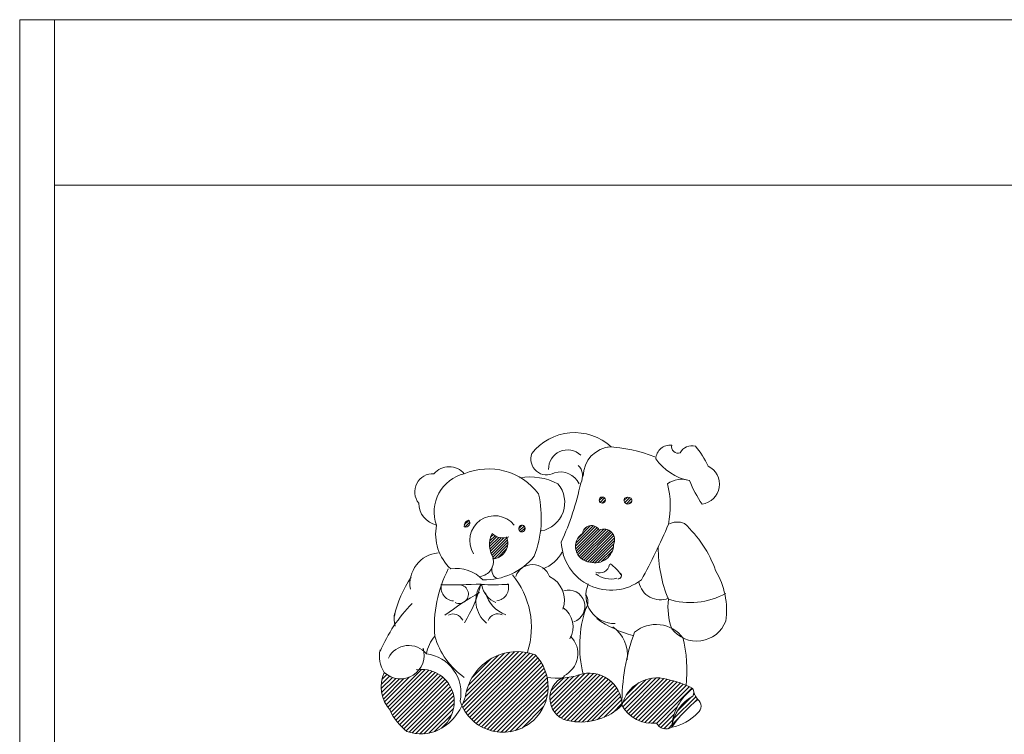
# Model space of a CAD drawing. Units: inches. Extents: x -17 to 1735, y -531 to 60.
# Tile 13 of 27: x 1734.65811 to 1734.68152, y -150.18312 to -150.16612. Entities that reach past the tile are written whole.
import ezdxf

# ---------------------------------------------------------------- set-up
doc = ezdxf.new("R2010")
doc.units = ezdxf.units.IN
doc.header["$MEASUREMENT"] = 0
doc.layers.add('A-FURN', color=242, linetype='Continuous', lineweight=18, true_color=0xcd2027)

# ---------------------------------------------------------------- blocks, each defined once
blk = doc.blocks.new('childrens_room_2')
for p, q in [((69.73591, 55.43419), (69.73591, 52.93419)), ((69.73591, 55.43419), (71.79591, 55.43419)), ((69.75691, 55.43419), (69.75691, 52.93419)), ((69.75691, 55.33419), (71.77791, 55.33419)), ((70.08595, 55.14364), (70.08806, 55.14576)), ((70.08652, 55.14255), (70.08916, 55.14519)), ((70.10093, 55.14362), (70.10296, 55.14564)), ((70.10141, 55.14243), (70.10447, 55.14548)), ((70.10235, 55.1417), (70.10548, 55.14483)), ((70.08769, 55.14205), (70.08967, 55.14404)), ((70.10389, 55.14157), (70.10561, 55.14328)), ((70.00446, 55.1289), (70.00723, 55.13166)), ((70.00492, 55.12768), (70.00776, 55.13053)), ((70.03738, 55.12677), (70.0394, 55.1288)), ((70.03775, 55.12548), (70.04054, 55.12827)), ((70.03867, 55.12473), (70.04115, 55.12721)), ((70.07163, 55.11599), (70.08361, 55.12796)), ((70.07175, 55.11443), (70.08464, 55.12732)), ((70.07184, 55.11786), (70.08237, 55.12839)), ((70.07284, 55.12053), (70.08079, 55.12848)), ((70.07662, 55.12598), (70.07827, 55.12763)), ((70.01971, 55.11745), (70.02412, 55.12186)), ((70.01974, 55.11582), (70.02535, 55.12142)), ((70.01987, 55.11928), (70.02302, 55.12243)), ((70.01993, 55.11433), (70.02673, 55.12114)), ((70.02024, 55.11297), (70.02833, 55.12106)), ((70.02037, 55.12145), (70.02202, 55.1231)), ((70.02064, 55.11171), (70.03014, 55.12121)), ((70.07206, 55.11308), (70.08548, 55.1265)), ((70.07253, 55.11188), (70.08674, 55.12609)), ((70.07312, 55.1108), (70.08874, 55.12642)), ((70.07383, 55.10984), (70.09025, 55.12625)), ((70.07464, 55.10898), (70.09149, 55.12583)), ((70.07555, 55.10823), (70.09255, 55.12522)), ((70.07658, 55.10758), (70.09344, 55.12445)), ((70.07772, 55.10706), (70.09419, 55.12353)), ((70.079, 55.10667), (70.09477, 55.12244)), ((70.08044, 55.10644), (70.09516, 55.12116)), ((70.02114, 55.11053), (70.0305, 55.1199)), ((70.02171, 55.10944), (70.03068, 55.11841)), ((70.02243, 55.10849), (70.0306, 55.11666)), ((70.08181, 55.10614), (70.09527, 55.1196)), ((70.08336, 55.10602), (70.09478, 55.11744)), ((70.08515, 55.10614), (70.09452, 55.11551)), ((70.02471, 55.10911), (70.02999, 55.11438)), ((70.08741, 55.10673), (70.09393, 55.11325)), ((70.00357, 55.01855), (70.03738, 55.05235)), ((70.00375, 55.02125), (70.03481, 55.05232)), ((70.00448, 55.01691), (70.03976, 55.0522)), ((70.00503, 55.02507), (70.032, 55.05204)), ((70.00547, 55.01537), (70.04198, 55.05189)), ((70.00579, 55.02836), (70.02885, 55.05142)), ((70.00655, 55.01392), (70.04408, 55.05145)), ((70.00696, 55.03206), (70.02515, 55.05025)), ((70.00771, 55.01255), (70.04605, 55.0509)), ((70.00896, 55.01127), (70.04771, 55.05002)), ((70.00938, 55.03701), (70.0202, 55.04783)), ((70.01029, 55.01007), (70.04888, 55.04866)), ((70.01171, 55.00895), (70.04997, 55.04722)), ((70.01321, 55.00793), (70.05097, 55.04569)), ((70.0148, 55.00698), (70.05189, 55.04407)), ((69.95473, 55.03553), (69.95771, 55.03851)), ((69.95583, 55.03916), (69.9563, 55.03963)), ((69.95722, 55.0203), (69.97853, 55.0416)), ((69.95821, 55.01876), (69.98093, 55.04148)), ((69.95932, 55.01733), (69.98309, 55.04111)), ((69.96023, 55.01571), (69.98506, 55.04055)), ((69.96111, 55.01406), (69.98688, 55.03983)), ((69.96207, 55.01249), (69.98855, 55.03896)), ((69.9631, 55.01099), (69.99009, 55.03798)), ((70.01649, 55.00614), (70.05271, 55.04237)), ((70.01827, 55.00539), (70.05343, 55.04056)), ((70.02017, 55.00476), (70.05405, 55.03863)), ((70.05654, 55.02088), (70.07405, 55.03838)), ((70.05717, 55.01897), (70.07735, 55.03916)), ((70.058, 55.01727), (70.08008, 55.03935)), ((70.05901, 55.01575), (70.08247, 55.03921)), ((70.06019, 55.0144), (70.08462, 55.03883)), ((70.06153, 55.01321), (70.08658, 55.03826)), ((69.95431, 55.03004), (69.96104, 55.03678)), ((69.95433, 55.0326), (69.95928, 55.03755)), ((69.95455, 55.02775), (69.96302, 55.03622)), ((69.95499, 55.02566), (69.96527, 55.03594)), ((69.9556, 55.02374), (69.96793, 55.03607)), ((69.95635, 55.02195), (69.97143, 55.03704)), ((69.96421, 55.00956), (69.99151, 55.03687)), ((69.96539, 55.00821), (69.99282, 55.03564)), ((69.96664, 55.00693), (69.99401, 55.0343)), ((69.96796, 55.00572), (69.99508, 55.03284)), ((70.02219, 55.00425), (70.05453, 55.03659)), ((70.02436, 55.00388), (70.05488, 55.0344)), ((70.02669, 55.00368), (70.05506, 55.03205)), ((70.05618, 55.02305), (70.07051, 55.03737)), ((70.0562, 55.0256), (70.06735, 55.03675)), ((70.05692, 55.02884), (70.06447, 55.0364)), ((70.06304, 55.01219), (70.08839, 55.03753)), ((70.06474, 55.01135), (70.09005, 55.03666)), ((70.06663, 55.01071), (70.09158, 55.03566)), ((70.06879, 55.01034), (70.09299, 55.03454)), ((70.07104, 55.01005), (70.09429, 55.0333)), ((70.07339, 55.00987), (70.09547, 55.03195)), ((70.10011, 55.02141), (70.11424, 55.03554)), ((70.10025, 55.01901), (70.11753, 55.03629)), ((70.10126, 55.01748), (70.1203, 55.03653)), ((70.10217, 55.02599), (70.10965, 55.03348)), ((70.10237, 55.01607), (70.12274, 55.03644)), ((70.10361, 55.01477), (70.12495, 55.03612)), ((70.10495, 55.01358), (70.127, 55.03563)), ((70.10641, 55.01251), (70.12905, 55.03515)), ((70.10798, 55.01155), (70.13105, 55.03462)), ((70.10968, 55.01072), (70.13299, 55.03403)), ((70.11152, 55.01002), (70.13489, 55.03339)), ((70.11352, 55.00949), (70.13673, 55.0327)), ((70.1157, 55.00914), (70.13853, 55.03197)), ((69.96935, 55.00458), (69.99604, 55.03126)), ((69.97108, 55.00377), (69.99686, 55.02955)), ((69.97306, 55.00322), (69.99753, 55.02769)), ((70.02923, 55.00369), (70.05502, 55.02948)), ((70.03206, 55.00399), (70.0547, 55.02663)), ((70.0759, 55.00985), (70.09653, 55.03048)), ((70.07861, 55.01003), (70.09746, 55.02888)), ((70.08158, 55.01047), (70.09827, 55.02716)), ((70.11813, 55.00904), (70.14027, 55.03118)), ((70.12069, 55.00907), (70.14198, 55.03036)), ((70.14276, 55.02607), (70.14348, 55.0268)), ((69.9752, 55.00283), (69.99804, 55.02567)), ((69.97754, 55.00264), (69.99834, 55.02344)), ((69.98012, 55.00268), (69.99838, 55.02095)), ((70.0353, 55.0047), (70.05395, 55.02335)), ((70.08492, 55.01128), (70.09892, 55.02528)), ((70.08888, 55.01271), (70.09941, 55.02323)), ((70.09436, 55.01565), (70.09968, 55.02097)), ((70.13088, 55.01166), (70.14436, 55.02514)), ((70.13299, 55.0163), (70.1418, 55.02511)), ((70.14358, 55.02183), (70.14541, 55.02366)), ((69.98305, 55.00308), (69.99803, 55.01806)), ((69.98657, 55.00407), (69.99694, 55.01444)), ((70.03934, 55.0062), (70.05241, 55.01927)), ((70.12175, 55.00759), (70.13309, 55.01893)), ((70.12317, 55.00648), (70.1313, 55.01461)), ((70.125, 55.00578), (70.13037, 55.01115)), ((70.12752, 55.00577), (70.1299, 55.00815)), ((70.13001, 55.00826), (70.13453, 55.01278))]:
    blk.add_line(p, q)
for centre, radius, start, end in [((70.07106, 55.15201), 0.03269, 47.56744, 142.1496), ((70.09417, 55.15831), 0.01786, 93.37661, 179.92184), ((70.08709, 55.08785), 0.08838, 68.42236, 87.41722), ((70.12888, 55.16833), 0.0088, 84.16796, 175.96386), ((70.13353, 55.17615), 0.00387, 165.93558, 290.16061), ((70.14204, 55.16872), 0.00811, 75.75386, 152.11841), ((70.10289, 55.14234), 0.05353, 24.30657, 39.76806), ((70.05427, 55.16875), 0.00962, 159.80669, 299.41128), ((70.06683, 55.16286), 0.01141, 45.88233, 182.2692), ((70.14635, 55.18708), 0.0319, 214.63102, 259.38614), ((69.99532, 55.15207), 0.01202, 40.3254, 139.6746), ((70.01904, 55.12494), 0.03783, 36.88695, 112.63886), ((70.06706, 55.15855), 0.00885, 330.59839, 45.68172), ((70.14652, 55.15345), 0.01208, 277.57709, 64.71768), ((69.98553, 55.14891), 0.01096, 86.76626, 218.74371), ((70.00995, 55.13682), 0.02367, 103.36537, 199.74983), ((70.04446, 55.12275), 0.03514, 61.90106, 100.43687), ((70.06265, 55.14875), 0.01219, 24.27878, 107.48315), ((70.04764, 55.14246), 0.0175, 280.50485, 40.14247), ((69.90549, 55.19016), 0.17306, 335.57302, 348.00674), ((70.13574, 55.14237), 0.01416, 70.50893, 126.96205), ((70.07581, 55.1404), 0.0531, 347.90233, 14.48761), ((70.20991, 55.1838), 0.07491, 202.01525, 214.40109), ((69.98657, 55.13298), 0.06442, 339.10374, 13.15578), ((70.0878, 55.14392), 0.00188, 115.18237, 21.2638), ((70.08777, 55.14384), 0.00194, 23.25863, 113.18754), ((70.1033, 55.14388), 0.00238, 148.79561, 31.20439), ((70.1033, 55.14154), 0.00411, 60.29008, 119.70992), ((69.99049, 55.14203), 0.01351, 179.95106, 257.97348), ((70.02279, 55.1195), 0.01499, 38.45263, 212.1028), ((70.01571, 55.12336), 0.02856, 168.97147, 227.27804), ((70.00803, 55.12842), 0.0036, 106.12208, 189.80326), ((70.00535, 55.13009), 0.00245, 249.25894, 46.6664), ((70.03954, 55.1267), 0.00216, 101.26279, 244.46967), ((70.03914, 55.12675), 0.00207, 255.10422, 90.62824), ((70.08124, 55.12301), 0.0055, 30.37045, 172.22212), ((69.81839, 55.25871), 0.33533, 330.91607, 337.29542), ((70.1331, 55.11955), 0.01111, 67.15156, 118.86656), ((70.09064, 55.07836), 0.06951, 19.26586, 47.70612), ((70.03485, 55.11698), 0.01515, 153.50993, 214.12765), ((70.02799, 55.13079), 0.00973, 226.46351, 290.94393), ((70.0211, 55.11799), 0.00959, 277.23711, 22.7381), ((70.08111, 55.1159), 0.00947, 124.08405, 265.60408), ((70.08879, 55.11993), 0.00649, 334.47929, 115.59175), ((70.09313, 55.11957), 0.03008, 181.86235, 307.50024), ((70.08348, 55.11718), 0.01116, 253.89883, 359.77278), ((70.20324, 55.115), 0.08161, 179.61744, 202.31721), ((69.99046, 55.09329), 0.01883, 95.36813, 189.55496), ((70.01676, 55.13442), 0.03867, 268.40803, 320.84993), ((70.04432, 55.1229), 0.02186, 290.19091, 331.75692), ((70.01287, 55.10688), 0.00917, 278.07246, 13.28765), ((70.02663, 55.10161), 0.00558, 149.91359, 239.98464), ((70.04573, 55.09407), 0.01084, 20.08269, 159.91731), ((70.08628, 55.10574), 0.00587, 246.55275, 352.10207), ((70.07455, 55.08074), 0.03059, 36.2381, 53.83293), ((70.02945, 55.05853), 0.06897, 145.81418, 167.13672), ((70.06185, 55.06778), 0.07544, 152.71223, 184.64057), ((69.99964, 55.08043), 0.02219, 43.69644, 98.57487), ((69.99529, 55.06703), 0.04971, 342.42, 39.74719), ((70.04885, 55.0833), 0.01613, 340.66235, 63.99998), ((70.09276, 55.1103), 0.01407, 231.22323, 286.18421), ((70.09736, 55.09832), 0.00204, 265.18933, 48.36203), ((70.11665, 55.0775), 0.04621, 351.64381, 31.00339), ((69.99254, 55.57151), 0.47882, 269.72587, 272.65535), ((69.99843, 55.091), 0.00799, 164.00776, 266.04303), ((70.00136, 55.08708), 0.00563, 244.15004, 93.95698), ((69.93641, 55.11292), 0.08059, 327.65523, 345.83593), ((70.02862, 55.08307), 0.01717, 144.95264, 231.46953), ((70.02222, 55.2529), 0.16015, 267.25738, 273.27551), ((70.02869, 55.0949), 0.01382, 190.26684, 248.40956), ((70.02325, 55.09103), 0.00799, 275.95697, 17.99224), ((70.09496, 55.08636), 0.01704, 156.20613, 272.35804), ((70.12291, 55.09693), 0.01326, 191.67005, 291.39822), ((70.11642, 54.90893), 0.20654, 119.82552, 126.7694), ((70.03583, 55.09268), 0.01915, 194.34108, 250.58121), ((70.06737, 55.07966), 0.0099, 289.68484, 106.29516), ((70.07225, 55.08255), 0.00691, 323.93269, 36.06731), ((70.14089, 55.12632), 0.04431, 252.73812, 299.0022), ((70.04386, 55.0132), 0.09849, 136.08462, 156.46965), ((70.16654, 55.07943), 0.03907, 173.27145, 199.78419), ((69.98152, 55.07287), 0.01947, 172.49519, 195.14241), ((69.99776, 55.06889), 0.00623, 23.09914, 118.06537), ((70.02469, 55.06896), 0.00623, 63.93463, 158.90086), ((70.05638, 55.06746), 0.01384, 328.15275, 56.27755), ((70.14484, 55.05603), 0.07066, 161.47853, 194.11081), ((70.12167, 55.12383), 0.0635, 234.12302, 256.04348), ((70.12026, 55.04849), 0.0203, 36.64265, 129.4253), ((70.14481, 55.07749), 0.0188, 216.90186, 339.08801), ((70.00368, 55.04701), 0.02247, 139.24246, 169.77568), ((70.03116, 55.07467), 0.04636, 196.27349, 234.86907), ((70.05827, 55.05115), 0.01479, 295.29465, 45.41874), ((70.08249, 55.0504), 0.02051, 351.7322, 55.42438), ((70.22362, 55.02128), 0.12391, 159.75091, 180.60607), ((69.97092, 55.04243), 0.01367, 38.83635, 153.82845), ((70.05801, 55.04094), 0.08096, 353.42744, 14.47269), ((69.97129, 55.04973), 0.01814, 167.8591, 213.14931), ((69.96591, 55.05025), 0.01433, 226.81434, 17.4152), ((69.97877, 55.02747), 0.02369, 347.92833, 83.21423), ((70.03653, 55.02068), 0.03169, 70.20494, 168.31718), ((70.02722, 55.03115), 0.02785, 313.07939, 43.97936), ((69.97576, 55.03115), 0.02148, 156.22792, 221.47729), ((69.97869, 55.02189), 0.01971, 302.22465, 99.46435), ((70.0609, 55.07773), 0.04148, 260.97704, 288.0398), ((70.08013, 55.01976), 0.01959, 0.61135, 109.02038), ((70.07009, 55.02424), 0.01396, 111.01364, 266.17459), ((70.12073, 55.01492), 0.02161, 73.91333, 166.47631), ((70.11402, 54.97479), 0.0622, 62.74823, 78.22322), ((69.97446, 55.03321), 0.03163, 297.77227, 348.84745), ((70.1612, 55.00476), 0.03148, 126.41748, 176.47666), ((70.13819, 55.0278), 0.00489, 332.06994, 27.93006), ((70.15637, 55.03257), 0.01413, 199.73505, 220.07171), ((70.02784, 55.03088), 0.02722, 197.89714, 312.52119), ((70.07492, 55.04523), 0.0354, 260.63456, 314.46709), ((70.11778, 55.02943), 0.02039, 207.6259, 277.97868), ((70.15425, 55.00385), 0.02464, 118.46656, 173.37564), ((70.19824, 54.95812), 0.08394, 128.8653, 144.64362), ((70.14226, 55.01941), 0.00524, 309.04303, 50.95697), ((69.98891, 55.02991), 0.032, 203.94632, 233.44262), ((70.1241, 55.03578), 0.02964, 281.03174, 316.38798), ((70.1263, 55.01195), 0.0063, 205.51602, 303.47239), ((69.97839, 55.02642), 0.0238, 248.98291, 297.03521)]:
    blk.add_arc(centre, radius, start, end)

msp = doc.modelspace()

# ---------------------------------------------------------------- block references
at = {"layer": 'A-FURN', "xscale": 0.0393700787401575, "yscale": 0.0393700787401575, "zscale": 0.0393700787401575}
msp.add_blockref('childrens_room_2', (1731.912601, -152.348565), dxfattribs=at)

doc.saveas('drawing.dxf')
